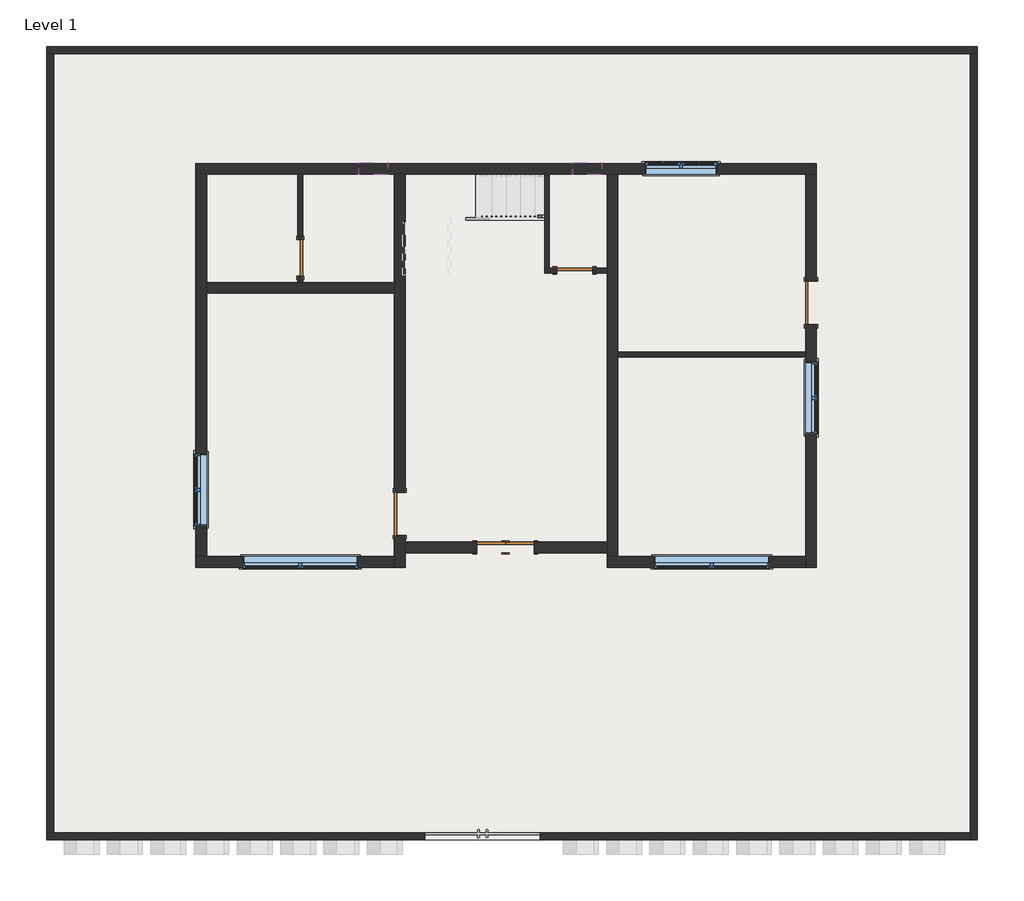
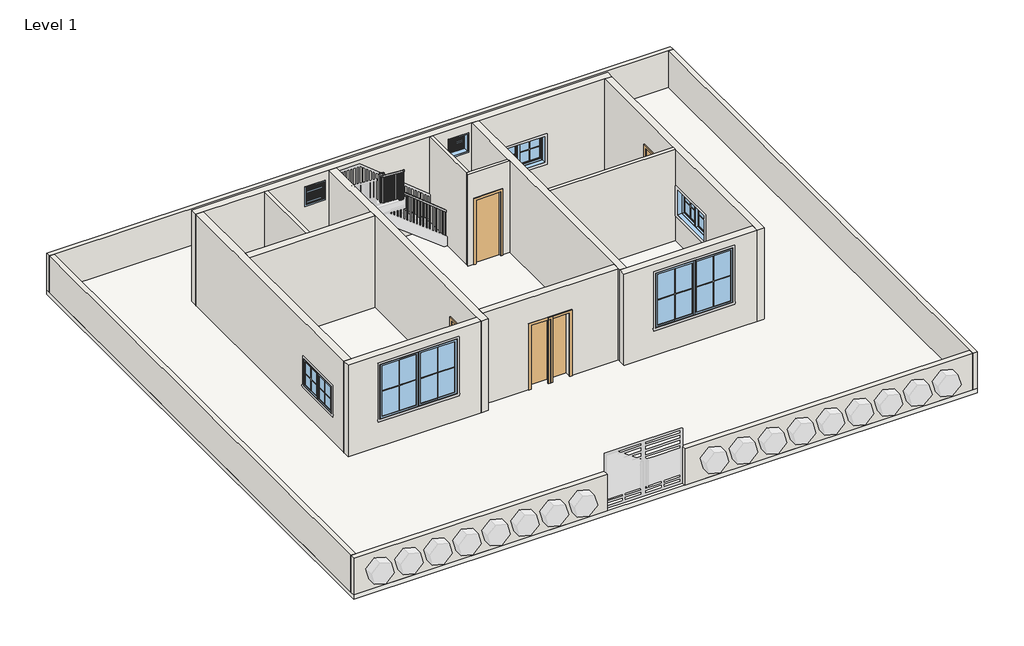
# One storey, part 1 of 2: 18 walls, 7 windows, 6 doors, 1 railing, 1 slab.
"""IFC4 building model written with IfcOpenShell, lengths in millimetres."""

from ifc_helpers import new_model, si_unit, frame, origin, origin_with_axes, place, context, project, spatial, polyline, outline, extrude, faceted_brep, transform, mapped, element, save
from components import single_flush_door_2_4a3212df, single_flush_door_2_0d3b4037, door_270f2424, door_aa9e95e7, single_flush_door_3_a90ba1ad, window_casement_double_c1d95f0f, window_casement_double_9ae172a2, window_f2d8fef0

model = new_model("IFC4")

# Units and contexts
model_context = context("Model", 3, world=origin())
ifc_project = project(units=[si_unit("LENGTHUNIT", "METRE", prefix="MILLI")], contexts=[model_context])

# Site, building, storey
site = spatial("IfcSite", under=ifc_project)
building = spatial("IfcBuilding", under=site)
storey = spatial("IfcBuildingStorey", under=building, Name="Level 1", Elevation=0.0)

# Doors
placement = place(None, origin())
single_flush_door_2_shape = single_flush_door_2_4a3212df(model_context)
element("IfcDoor", 1, ObjectType="Single-Flush : DOOR 2'", at=placement, inside=storey, context=model_context, shape_type="MappedRepresentation", body=[
    mapped(single_flush_door_2_shape, transform((-1572.7415084, -2604.3618005, 0.0), x_axis=(-1.0, 0.0, 0.0), y_axis=(0.0, -1.0, 0.0), z_axis=(0.0, 0.0, 1.0))),
])
single_flush_door_2_2_shape = single_flush_door_2_0d3b4037(model_context)
element("IfcDoor", 2, ObjectType="Single-Flush : DOOR 2'", at=placement, inside=storey, context=model_context, shape_type="MappedRepresentation", body=[
    mapped(single_flush_door_2_2_shape, transform((-963.1415084, -2604.3618005, 0.0), x_axis=(1.0, 0.0, 0.0), y_axis=(0.0, 1.0, 0.0), z_axis=(0.0, 0.0, 1.0))),
])
door_shape = door_270f2424(model_context)
element("IfcDoor", 3, ObjectType="Single-Flush : DOOR 2'6\"", at=placement, inside=storey, context=model_context, shape_type="MappedRepresentation", body=[
    mapped(door_shape, transform((-5598.6415084, 3517.0381995, 0.0), x_axis=(0.0, -1.0, 0.0), y_axis=(1.0, 0.0, 0.0), z_axis=(0.0, 0.0, 1.0))),
])
door_2_shape = door_aa9e95e7(model_context)
element("IfcDoor", 4, ObjectType="Single-Flush : DOOR 2'6\"", at=placement, inside=storey, context=model_context, shape_type="MappedRepresentation", body=[
    mapped(door_2_shape, transform((192.5584916, 3250.3381995, 0.0), x_axis=(-1.0, 0.0, 0.0), y_axis=(0.0, -1.0, 0.0), z_axis=(0.0, 0.0, 1.0))),
])
single_flush_door_3_shape = single_flush_door_3_a90ba1ad(model_context)
element("IfcDoor", 5, ObjectType="Single-Flush : DOOR 3'", at=placement, inside=storey, context=model_context, shape_type="MappedRepresentation", body=[
    mapped(single_flush_door_3_shape, transform((-3503.1415084, -1893.1618005, 0.0), x_axis=(0.0, -1.0, 0.0), y_axis=(1.0, 0.0, 0.0), z_axis=(0.0, 0.0, 1.0))),
])
element("IfcDoor", 6, ObjectType="Single-Flush : DOOR 3'", at=placement, inside=storey, context=model_context, shape_type="MappedRepresentation", body=[
    mapped(single_flush_door_3_shape, transform((5183.6584916, 2564.5381995, 0.0), x_axis=(0.0, -1.0, 0.0), y_axis=(1.0, 0.0, 0.0), z_axis=(0.0, 0.0, 1.0))),
])

# Railing
element("IfcRailing", 7, ObjectType="Handrail - Rectangular", at=placement, inside=storey, context=model_context, shape_type="SolidModel", body=[
    faceted_brep([(-442.4415084, 4368.3146777, 1148.8615385), (-442.4415084, 4368.3146777, 1083.5609717), (-442.4415084, 4419.1146777, 1083.5609717), (-442.4415084, 4419.1146777, 1148.8615385), (-2398.2415084, 4368.3146777, 2728.5461538), (-2449.0415084, 4368.3146777, 2704.2763563), (-2449.0415084, 4419.1146777, 2704.2763563), (-2398.2415084, 4419.1146777, 2728.5461538), (-2398.2415084, 4368.3146777, 3083.1511426), (-2449.0415084, 4368.3146777, 3032.3511426), (-2449.0415084, 4419.1146777, 3032.3511426), (-2398.2415084, 4419.1146777, 3083.1511426), (-2474.4415084, 4368.3146777, 3083.1511426), (-2474.4415084, 4368.3146777, 3032.3511426), (-2525.2415084, 4419.1146777, 3032.3511426), (-2525.2415084, 4419.1146777, 3083.1511426), (-2474.4415084, 4292.1146777, 3083.1511426), (-2474.4415084, 4274.8407094, 3032.3511426), (-2525.2415084, 4274.8407094, 3032.3511426), (-2525.2415084, 4292.1146777, 3083.1511426), (-2474.4415084, 3148.7383287, 3962.4), (-2525.2415084, 3148.7383287, 3962.4), (-2525.2415084, 3148.7383287, 3898.3164325), (-2474.4415084, 3148.7383287, 3898.3164325)], [[[0, 1, 2, 3]], [[1, 0, 4, 5]], [[2, 1, 5, 6]], [[3, 2, 6, 7]], [[0, 3, 7, 4]], [[5, 4, 8, 9]], [[6, 5, 9, 10]], [[7, 6, 10, 11]], [[4, 7, 11, 8]], [[9, 8, 12, 13]], [[10, 9, 13, 14]], [[11, 10, 14, 15]], [[8, 11, 15, 12]], [[13, 12, 16, 17]], [[14, 13, 17, 18]], [[15, 14, 18, 19]], [[12, 15, 19, 16]], [[20, 21, 22, 23]], [[17, 16, 20, 23]], [[18, 17, 23, 22]], [[19, 18, 22, 21]], [[16, 19, 21, 20]]]),
    extrude(outline(polyline([(3184.0396777, 3871.1699284), (3184.0396777, 2813.5384615), (3164.9896777, 2813.5384615), (3164.9896777, 3885.8192525), (3184.0396777, 3871.1699284)])), frame((-2509.3665084, 0.0, 0.0), z_axis=(1.0, 0.0, 0.0), x_axis=(0.0, 1.0, 0.0)), (0.0, 0.0, 1.0), 19.05),
    extrude(outline(polyline([(3285.6396777, 3793.0401997), (3285.6396777, 2813.5384615), (3266.5896777, 2813.5384615), (3266.5896777, 3807.6895238), (3285.6396777, 3793.0401997)])), frame((-2509.3665084, 0.0, 0.0), z_axis=(1.0, 0.0, 0.0), x_axis=(0.0, 1.0, 0.0)), (0.0, 0.0, 1.0), 19.05),
    extrude(outline(polyline([(3387.2396777, 3714.910471), (3387.2396777, 2813.5384615), (3368.1896777, 2813.5384615), (3368.1896777, 3729.5597952), (3387.2396777, 3714.910471)])), frame((-2509.3665084, 0.0, 0.0), z_axis=(1.0, 0.0, 0.0), x_axis=(0.0, 1.0, 0.0)), (0.0, 0.0, 1.0), 19.05),
    extrude(outline(polyline([(3488.8396777, 3636.9254473), (3488.8396777, 2579.0769231), (3469.7896777, 2579.0769231), (3469.7896777, 3651.5747714), (3488.8396777, 3636.9254473)])), frame((-2509.3665084, 0.0, 0.0), z_axis=(1.0, 0.0, 0.0), x_axis=(0.0, 1.0, 0.0)), (0.0, 0.0, 1.0), 19.05),
    extrude(outline(polyline([(3590.4396777, 3558.7957187), (3590.4396777, 2579.0769231), (3571.3896777, 2579.0769231), (3571.3896777, 3573.4450428), (3590.4396777, 3558.7957187)])), frame((-2509.3665084, 0.0, 0.0), z_axis=(1.0, 0.0, 0.0), x_axis=(0.0, 1.0, 0.0)), (0.0, 0.0, 1.0), 19.05),
    extrude(outline(polyline([(3692.0396777, 3480.66599), (3692.0396777, 2579.0769231), (3672.9896777, 2579.0769231), (3672.9896777, 3495.3153141), (3692.0396777, 3480.66599)])), frame((-2509.3665084, 0.0, 0.0), z_axis=(1.0, 0.0, 0.0), x_axis=(0.0, 1.0, 0.0)), (0.0, 0.0, 1.0), 19.05),
    extrude(outline(polyline([(3793.6396777, 3402.4639089), (3793.6396777, 2344.6153846), (3774.5896777, 2344.6153846), (3774.5896777, 3417.113233), (3793.6396777, 3402.4639089)])), frame((-2509.3665084, 0.0, 0.0), z_axis=(1.0, 0.0, 0.0), x_axis=(0.0, 1.0, 0.0)), (0.0, 0.0, 1.0), 19.05),
    extrude(outline(polyline([(3895.2396777, 3324.3341802), (3895.2396777, 2344.6153846), (3876.1896777, 2344.6153846), (3876.1896777, 3338.9835043), (3895.2396777, 3324.3341802)])), frame((-2509.3665084, 0.0, 0.0), z_axis=(1.0, 0.0, 0.0), x_axis=(0.0, 1.0, 0.0)), (0.0, 0.0, 1.0), 19.05),
    extrude(outline(polyline([(3996.8396777, 3246.2044515), (3996.8396777, 2344.6153846), (3977.7896777, 2344.6153846), (3977.7896777, 3260.8537757), (3996.8396777, 3246.2044515)])), frame((-2509.3665084, 0.0, 0.0), z_axis=(1.0, 0.0, 0.0), x_axis=(0.0, 1.0, 0.0)), (0.0, 0.0, 1.0), 19.05),
    extrude(outline(polyline([(4098.4396777, 3168.0023704), (4098.4396777, 2110.1538462), (4079.3896777, 2110.1538462), (4079.3896777, 3182.6516945), (4098.4396777, 3168.0023704)])), frame((-2509.3665084, 0.0, 0.0), z_axis=(1.0, 0.0, 0.0), x_axis=(0.0, 1.0, 0.0)), (0.0, 0.0, 1.0), 19.05),
    extrude(outline(polyline([(4200.0396777, 3089.8726417), (4200.0396777, 2110.1538462), (4180.9896777, 2110.1538462), (4180.9896777, 3104.5219659), (4200.0396777, 3089.8726417)])), frame((-2509.3665084, 0.0, 0.0), z_axis=(1.0, 0.0, 0.0), x_axis=(0.0, 1.0, 0.0)), (0.0, 0.0, 1.0), 19.05),
    extrude(outline(polyline([(4301.6396777, 3011.7429131), (4301.6396777, 2110.1538462), (4282.5896777, 2110.1538462), (4282.5896777, 3026.3922372), (4301.6396777, 3011.7429131)])), frame((-2509.3665084, 0.0, 0.0), z_axis=(1.0, 0.0, 0.0), x_axis=(0.0, 1.0, 0.0)), (0.0, 0.0, 1.0), 19.05),
    extrude(outline(polyline([(-2464.9165084, 4384.1896777), (-2483.9665084, 4384.1896777), (-2483.9665084, 4403.2396777), (-2464.9165084, 4403.2396777), (-2464.9165084, 4384.1896777)])), frame((0.0, 0.0, 1875.6923077), z_axis=(0.0, 0.0, 1.0), x_axis=(1.0, 0.0, 0.0)), (0.0, 0.0, 1.0), 1156.658835),
    extrude(outline(polyline([(2650.4234717, -2382.3665084), (1641.2307692, -2382.3665084), (1641.2307692, -2363.3165084), (2635.0369332, -2363.3165084), (2650.4234717, -2382.3665084)])), frame((0.0, 4384.1896777, 0.0), z_axis=(0.0, 1.0, 0.0), x_axis=(0.0, 0.0, 1.0)), (0.0, 0.0, 1.0), 19.05),
    extrude(outline(polyline([(2568.3619332, -2280.7665084), (1641.2307692, -2280.7665084), (1641.2307692, -2261.7165084), (2552.9753947, -2261.7165084), (2568.3619332, -2280.7665084)])), frame((0.0, 4384.1896777, 0.0), z_axis=(0.0, 1.0, 0.0), x_axis=(0.0, 0.0, 1.0)), (0.0, 0.0, 1.0), 19.05),
    extrude(outline(polyline([(2486.3003947, -2179.1665084), (1641.2307692, -2179.1665084), (1641.2307692, -2160.1165084), (2470.9138563, -2160.1165084), (2486.3003947, -2179.1665084)])), frame((0.0, 4384.1896777, 0.0), z_axis=(0.0, 1.0, 0.0), x_axis=(0.0, 0.0, 1.0)), (0.0, 0.0, 1.0), 19.05),
    extrude(outline(polyline([(2404.2388563, -2077.5665084), (1406.7692308, -2077.5665084), (1406.7692308, -2058.5165084), (2388.8523178, -2058.5165084), (2404.2388563, -2077.5665084)])), frame((0.0, 4384.1896777, 0.0), z_axis=(0.0, 1.0, 0.0), x_axis=(0.0, 0.0, 1.0)), (0.0, 0.0, 1.0), 19.05),
    extrude(outline(polyline([(2322.1773178, -1975.9665084), (1406.7692308, -1975.9665084), (1406.7692308, -1956.9165084), (2306.7907794, -1956.9165084), (2322.1773178, -1975.9665084)])), frame((0.0, 4384.1896777, 0.0), z_axis=(0.0, 1.0, 0.0), x_axis=(0.0, 0.0, 1.0)), (0.0, 0.0, 1.0), 19.05),
    extrude(outline(polyline([(2240.1157794, -1874.3665084), (1406.7692308, -1874.3665084), (1406.7692308, -1855.3165084), (2224.7292409, -1855.3165084), (2240.1157794, -1874.3665084)])), frame((0.0, 4384.1896777, 0.0), z_axis=(0.0, 1.0, 0.0), x_axis=(0.0, 0.0, 1.0)), (0.0, 0.0, 1.0), 19.05),
    extrude(outline(polyline([(2158.0542409, -1772.7665084), (1172.3076923, -1772.7665084), (1172.3076923, -1753.7165084), (2142.6677024, -1753.7165084), (2158.0542409, -1772.7665084)])), frame((0.0, 4384.1896777, 0.0), z_axis=(0.0, 1.0, 0.0), x_axis=(0.0, 0.0, 1.0)), (0.0, 0.0, 1.0), 19.05),
    extrude(outline(polyline([(2075.9927024, -1671.1665084), (1172.3076923, -1671.1665084), (1172.3076923, -1652.1165084), (2060.606164, -1652.1165084), (2075.9927024, -1671.1665084)])), frame((0.0, 4384.1896777, 0.0), z_axis=(0.0, 1.0, 0.0), x_axis=(0.0, 0.0, 1.0)), (0.0, 0.0, 1.0), 19.05),
    extrude(outline(polyline([(1993.931164, -1569.5665084), (1172.3076923, -1569.5665084), (1172.3076923, -1550.5165084), (1978.5446255, -1550.5165084), (1993.931164, -1569.5665084)])), frame((0.0, 4384.1896777, 0.0), z_axis=(0.0, 1.0, 0.0), x_axis=(0.0, 0.0, 1.0)), (0.0, 0.0, 1.0), 19.05),
    extrude(outline(polyline([(1911.8696255, -1467.9665084), (937.8461538, -1467.9665084), (937.8461538, -1448.9165084), (1896.4830871, -1448.9165084), (1911.8696255, -1467.9665084)])), frame((0.0, 4384.1896777, 0.0), z_axis=(0.0, 1.0, 0.0), x_axis=(0.0, 0.0, 1.0)), (0.0, 0.0, 1.0), 19.05),
    extrude(outline(polyline([(1829.8080871, -1366.3665084), (937.8461538, -1366.3665084), (937.8461538, -1347.3165084), (1814.4215486, -1347.3165084), (1829.8080871, -1366.3665084)])), frame((0.0, 4384.1896777, 0.0), z_axis=(0.0, 1.0, 0.0), x_axis=(0.0, 0.0, 1.0)), (0.0, 0.0, 1.0), 19.05),
    extrude(outline(polyline([(1747.7465486, -1264.7665084), (937.8461538, -1264.7665084), (937.8461538, -1245.7165084), (1732.3600101, -1245.7165084), (1747.7465486, -1264.7665084)])), frame((0.0, 4384.1896777, 0.0), z_axis=(0.0, 1.0, 0.0), x_axis=(0.0, 0.0, 1.0)), (0.0, 0.0, 1.0), 19.05),
    extrude(outline(polyline([(1665.6850101, -1163.1665084), (703.3846154, -1163.1665084), (703.3846154, -1144.1165084), (1650.2984717, -1144.1165084), (1665.6850101, -1163.1665084)])), frame((0.0, 4384.1896777, 0.0), z_axis=(0.0, 1.0, 0.0), x_axis=(0.0, 0.0, 1.0)), (0.0, 0.0, 1.0), 19.05),
    extrude(outline(polyline([(1583.6234717, -1061.5665084), (703.3846154, -1061.5665084), (703.3846154, -1042.5165084), (1568.2369332, -1042.5165084), (1583.6234717, -1061.5665084)])), frame((0.0, 4384.1896777, 0.0), z_axis=(0.0, 1.0, 0.0), x_axis=(0.0, 0.0, 1.0)), (0.0, 0.0, 1.0), 19.05),
    extrude(outline(polyline([(1501.5619332, -959.9665084), (703.3846154, -959.9665084), (703.3846154, -940.9165084), (1486.1753947, -940.9165084), (1501.5619332, -959.9665084)])), frame((0.0, 4384.1896777, 0.0), z_axis=(0.0, 1.0, 0.0), x_axis=(0.0, 0.0, 1.0)), (0.0, 0.0, 1.0), 19.05),
    extrude(outline(polyline([(1419.5003947, -858.3665084), (468.9230769, -858.3665084), (468.9230769, -839.3165084), (1404.1138563, -839.3165084), (1419.5003947, -858.3665084)])), frame((0.0, 4384.1896777, 0.0), z_axis=(0.0, 1.0, 0.0), x_axis=(0.0, 0.0, 1.0)), (0.0, 0.0, 1.0), 19.05),
    extrude(outline(polyline([(1337.4388563, -756.7665084), (468.9230769, -756.7665084), (468.9230769, -737.7165084), (1322.0523178, -737.7165084), (1337.4388563, -756.7665084)])), frame((0.0, 4384.1896777, 0.0), z_axis=(0.0, 1.0, 0.0), x_axis=(0.0, 0.0, 1.0)), (0.0, 0.0, 1.0), 19.05),
    extrude(outline(polyline([(1255.3773178, -655.1665084), (468.9230769, -655.1665084), (468.9230769, -636.1165084), (1239.9907794, -636.1165084), (1255.3773178, -655.1665084)])), frame((0.0, 4384.1896777, 0.0), z_axis=(0.0, 1.0, 0.0), x_axis=(0.0, 0.0, 1.0)), (0.0, 0.0, 1.0), 19.05),
    extrude(outline(polyline([(1173.3157794, -553.5665084), (234.4615385, -553.5665084), (234.4615385, -534.5165084), (1157.9292409, -534.5165084), (1173.3157794, -553.5665084)])), frame((0.0, 4384.1896777, 0.0), z_axis=(0.0, 1.0, 0.0), x_axis=(0.0, 0.0, 1.0)), (0.0, 0.0, 1.0), 19.05),
    extrude(outline(polyline([(-2490.3165084, 4384.1896777), (-2509.3665084, 4384.1896777), (-2509.3665084, 4403.2396777), (-2490.3165084, 4403.2396777), (-2490.3165084, 4384.1896777)])), frame((0.0, 0.0, 1875.6923077), z_axis=(0.0, 0.0, 1.0), x_axis=(1.0, 0.0, 0.0)), (0.0, 0.0, 1.0), 1156.658835),
    extrude(outline(polyline([(3167.7883287, 3883.6671084), (3167.7883287, 2813.5384615), (3148.7383287, 2813.5384615), (3148.7383287, 3898.3164325), (3167.7883287, 3883.6671084)])), frame((-2509.3665084, 0.0, 0.0), z_axis=(1.0, 0.0, 0.0), x_axis=(0.0, 1.0, 0.0)), (0.0, 0.0, 1.0), 19.05),
    extrude(outline(polyline([(1098.9475101, -461.4915084), (234.4615385, -461.4915084), (234.4615385, -442.4415084), (1083.5609717, -442.4415084), (1098.9475101, -461.4915084)])), frame((0.0, 4384.1896777, 0.0), z_axis=(0.0, 1.0, 0.0), x_axis=(0.0, 0.0, 1.0)), (0.0, 0.0, 1.0), 19.05),
])

# Slab
element("IfcSlab", 8, ObjectType="FLOOR 6\"", at=placement, inside=storey, context=model_context, shape_type="SweptSolid", body=[
    extrude(outline(polyline([(8700.0547931, 7982.1774536), (8700.0547931, -8781.8225464), (-10959.5452069, -8781.8225464), (-10959.5452069, 7982.1774536), (8700.0547931, 7982.1774536)])), frame((0.0, 0.0, -152.4), z_axis=(0.0, 0.0, 1.0), x_axis=(1.0, 0.0, 0.0)), (0.0, 0.0, 1.0), 152.4),
])

# Walls
element("IfcWall", 9, ObjectType="CMD 6\"", at=placement, inside=storey, context=model_context, shape_type="Brep", body=[
    faceted_brep([(-10959.5452069, 7829.7774536, 0.0), (-10807.1452069, 7829.7774536, 0.0), (8547.6547931, 7829.7774536, 0.0), (8700.0547931, 7829.7774536, 0.0), (8700.0547931, 7829.7774536, 1219.2), (8547.6547931, 7829.7774536, 1219.2), (-10807.1452069, 7829.7774536, 1219.2), (-10959.5452069, 7829.7774536, 1219.2), (-10959.5452069, 7982.1774536, 0.0), (-10959.5452069, 7982.1774536, 1219.2), (8700.0547931, 7982.1774536, 1219.2), (8700.0547931, 7982.1774536, 0.0)], [[[0, 1, 2, 3, 4, 5, 6, 7]], [[8, 9, 10, 11]], [[3, 2, 1, 0, 8, 11]], [[7, 6, 5, 4, 10, 9]], [[4, 3, 11, 10]], [[0, 7, 9, 8]]]),
])
element("IfcWall", 10, ObjectType="CMD 6\"", at=placement, inside=storey, context=model_context, shape_type="Brep", body=[
    faceted_brep([(8547.6547931, 7829.7774536, 0.0), (8547.6547931, -8629.4225464, 0.0), (8547.6547931, -8781.8225464, 0.0), (8547.6547931, -8781.8225464, 1219.2), (8547.6547931, -8629.4225464, 1219.2), (8547.6547931, 7829.7774536, 1219.2), (8700.0547931, 7829.7774536, 0.0), (8700.0547931, 7829.7774536, 1219.2), (8700.0547931, -8781.8225464, 1219.2), (8700.0547931, -8781.8225464, 0.0)], [[[0, 1, 2, 3, 4, 5]], [[6, 7, 8, 9]], [[2, 1, 0, 6, 9]], [[5, 4, 3, 8, 7]], [[0, 5, 7, 6]], [[3, 2, 9, 8]]]),
])
element("IfcWall", 11, ObjectType="CMD 6\"", at=placement, inside=storey, context=model_context, shape_type="SweptSolid", body=[
    extrude(outline(polyline([(-531.3415084, -8629.4225464), (8547.6547931, -8629.4225464), (8547.6547931, -8781.8225464), (-531.3415084, -8781.8225464), (-531.3415084, -8629.4225464)])), origin_with_axes(), (0.0, 0.0, 1.0), 1219.2),
])
element("IfcWall", 12, ObjectType="CMD 6\"", at=placement, inside=storey, context=model_context, shape_type="SweptSolid", body=[
    extrude(outline(polyline([(-10807.1452069, 7829.7774536), (-10807.1452069, -8629.4225464), (-10959.5452069, -8629.4225464), (-10959.5452069, 7829.7774536), (-10807.1452069, 7829.7774536)])), origin_with_axes(), (0.0, 0.0, 1.0), 1219.2),
])
element("IfcWall", 13, ObjectType="CMD 6\"", at=placement, inside=storey, context=model_context, shape_type="Brep", body=[
    faceted_brep([(-2969.7415084, -8629.4225464, 0.0), (-10807.1452069, -8629.4225464, 0.0), (-10959.5452069, -8629.4225464, 0.0), (-10959.5452069, -8629.4225464, 1219.2), (-10807.1452069, -8629.4225464, 1219.2), (-2969.7415084, -8629.4225464, 1219.2), (-2969.7415084, -8781.8225464, 0.0), (-2969.7415084, -8781.8225464, 1219.2), (-10959.5452069, -8781.8225464, 1219.2), (-10959.5452069, -8781.8225464, 0.0)], [[[0, 1, 2, 3, 4, 5]], [[6, 7, 8, 9]], [[2, 1, 0, 6, 9]], [[5, 4, 3, 8, 7]], [[0, 5, 7, 6]], [[3, 2, 9, 8]]]),
])
element("IfcWall", 14, ObjectType="WALL 4\"", at=placement, inside=storey, context=model_context, shape_type="SweptSolid", body=[
    extrude(outline(polyline([(3136.0381995, 2133.6), (3136.0381995, 0.0), (2996.3381995, 0.0), (2996.3381995, 3048.0), (5282.3381995, 3048.0), (5282.3381995, 0.0), (3898.0381995, 0.0), (3898.0381995, 2133.6), (3136.0381995, 2133.6)])), frame((-5649.4415084, 0.0, 0.0), z_axis=(1.0, 0.0, 0.0), x_axis=(0.0, 1.0, 0.0)), (0.0, 0.0, 1.0), 101.6),
])
element("IfcWall", 15, ObjectType="WALL 4\"", at=placement, inside=storey, context=model_context, shape_type="Brep", body=[
    faceted_brep([(-188.4415084, 3301.1381995, 2133.6), (-188.4415084, 3301.1381995, 0.0), (-340.8415084, 3301.1381995, 0.0), (-442.4415084, 3301.1381995, 0.0), (-442.4415084, 3301.1381995, 3048.0), (-340.8415084, 3301.1381995, 3048.0), (878.3584916, 3301.1381995, 3048.0), (878.3584916, 3301.1381995, 0.0), (573.5584916, 3301.1381995, 0.0), (573.5584916, 3301.1381995, 2133.6), (-442.4415084, 3199.5381995, 0.0), (-188.4415084, 3199.5381995, 0.0), (-188.4415084, 3199.5381995, 2133.6), (573.5584916, 3199.5381995, 2133.6), (573.5584916, 3199.5381995, 0.0), (878.3584916, 3199.5381995, 0.0), (878.3584916, 3199.5381995, 3048.0), (-442.4415084, 3199.5381995, 3048.0)], [[[0, 1, 2, 3, 4, 5, 6, 7, 8, 9]], [[10, 11, 12, 13, 14, 15, 16, 17]], [[8, 7, 15, 14]], [[3, 2, 1, 11, 10]], [[7, 6, 16, 15]], [[4, 3, 10, 17]], [[12, 11, 1, 0]], [[13, 12, 0, 9]], [[14, 13, 9, 8]], [[6, 5, 4, 17, 16]]]),
])
element("IfcWall", 16, ObjectType="WALL 4\"", at=placement, inside=storey, context=model_context, shape_type="Brep", body=[
    faceted_brep([(-340.8415084, 3301.1381995, 0.0), (-340.8415084, 5282.3381995, 0.0), (-340.8415084, 5282.3381995, 3048.0), (-340.8415084, 3301.1381995, 3048.0), (-442.4415084, 3301.1381995, 0.0), (-442.4415084, 3301.1381995, 3048.0), (-442.4415084, 4317.5146777, 3048.0), (-442.4415084, 5282.3381995, 3048.0), (-442.4415084, 5282.3381995, 0.0)], [[[0, 1, 2, 3]], [[4, 5, 6, 7, 8]], [[1, 0, 4, 8]], [[0, 3, 5, 4]], [[2, 1, 8, 7]], [[3, 2, 7, 6, 5]]]),
])
element("IfcWall", 17, ObjectType="WALL 4\"", at=placement, inside=storey, context=model_context, shape_type="SweptSolid", body=[
    extrude(outline(polyline([(1106.9584916, 1523.1381995), (5069.3584916, 1523.1381995), (5069.3584916, 1421.5381995), (1106.9584916, 1421.5381995), (1106.9584916, 1523.1381995)])), origin_with_axes(), (0.0, 0.0, 1.0), 3048.0),
])
element("IfcWall", 18, ObjectType="WALL 9\"", at=placement, inside=storey, context=model_context, shape_type="Brep", body=[
    faceted_brep([(-7808.4415084, 5282.3381995, 0.0), (-7579.8415084, 5282.3381995, 0.0), (-5649.4415084, 5282.3381995, 0.0), (-5547.8415084, 5282.3381995, 0.0), (-3617.4415084, 5282.3381995, 0.0), (-3388.8415084, 5282.3381995, 0.0), (-442.4415084, 5282.3381995, 0.0), (-340.8415084, 5282.3381995, 0.0), (878.3584916, 5282.3381995, 0.0), (1106.9584916, 5282.3381995, 0.0), (5069.3584916, 5282.3381995, 0.0), (5297.9584916, 5282.3381995, 0.0), (5297.9584916, 5282.3381995, 3048.0), (5069.3584916, 5282.3381995, 3048.0), (1106.9584916, 5282.3381995, 3048.0), (878.3584916, 5282.3381995, 3048.0), (-340.8415084, 5282.3381995, 3048.0), (-442.4415084, 5282.3381995, 3048.0), (-3388.8415084, 5282.3381995, 3048.0), (-3617.4415084, 5282.3381995, 3048.0), (-5547.8415084, 5282.3381995, 3048.0), (-5649.4415084, 5282.3381995, 3048.0), (-7579.8415084, 5282.3381995, 3048.0), (-7808.4415084, 5282.3381995, 3048.0), (3202.4584916, 5282.3381995, 1828.8), (3202.4584916, 5282.3381995, 914.4), (1678.4584916, 5282.3381995, 914.4), (1678.4584916, 5282.3381995, 1828.8), (154.4584916, 5282.3381995, 2743.2), (764.0584916, 5282.3381995, 2743.2), (764.0584916, 5282.3381995, 2133.6), (154.4584916, 5282.3381995, 2133.6), (-3757.1415084, 5282.3381995, 2743.2), (-3757.1415084, 5282.3381995, 2133.6), (-4366.7415084, 5282.3381995, 2133.6), (-4366.7415084, 5282.3381995, 2743.2), (-7808.4415084, 5510.9381995, 0.0), (-7808.4415084, 5510.9381995, 3048.0), (5297.9584916, 5510.9381995, 3048.0), (5297.9584916, 5510.9381995, 0.0), (3202.4584916, 5510.9381995, 1828.8), (1678.4584916, 5510.9381995, 1828.8), (1678.4584916, 5510.9381995, 914.4), (3202.4584916, 5510.9381995, 914.4), (154.4584916, 5510.9381995, 2743.2), (154.4584916, 5510.9381995, 2133.6), (764.0584916, 5510.9381995, 2133.6), (764.0584916, 5510.9381995, 2743.2), (-3757.1415084, 5510.9381995, 2743.2), (-4366.7415084, 5510.9381995, 2743.2), (-4366.7415084, 5510.9381995, 2133.6), (-3757.1415084, 5510.9381995, 2133.6)], [[[0, 1, 2, 3, 4, 5, 6, 7, 8, 9, 10, 11, 12, 13, 14, 15, 16, 17, 18, 19, 20, 21, 22, 23], [24, 25, 26, 27], [28, 29, 30, 31], [32, 33, 34, 35]], [[36, 37, 38, 39], [40, 41, 42, 43], [44, 45, 46, 47], [48, 49, 50, 51]], [[11, 10, 9, 8, 7, 6, 5, 4, 3, 2, 1, 0, 36, 39]], [[23, 22, 21, 20, 19, 18, 17, 16, 15, 14, 13, 12, 38, 37]], [[12, 11, 39, 38]], [[0, 23, 37, 36]], [[25, 24, 40, 43]], [[26, 25, 43, 42]], [[27, 26, 42, 41]], [[24, 27, 41, 40]], [[45, 44, 28, 31]], [[46, 45, 31, 30]], [[47, 46, 30, 29]], [[44, 47, 29, 28]], [[33, 32, 48, 51]], [[34, 33, 51, 50]], [[35, 34, 50, 49]], [[32, 35, 49, 48]]]),
])
element("IfcWall", 19, ObjectType="WALL 9\"", at=placement, inside=storey, context=model_context, shape_type="Brep", body=[
    faceted_brep([(5069.3584916, 2107.3381995, 2133.6), (5069.3584916, 2107.3381995, 0.0), (5069.3584916, 1523.1381995, 0.0), (5069.3584916, 1421.5381995, 0.0), (5069.3584916, -2794.8618005, 0.0), (5069.3584916, -3023.4618005, 0.0), (5069.3584916, -3023.4618005, 3048.0), (5069.3584916, -2794.8618005, 3048.0), (5069.3584916, 1421.5381995, 3048.0), (5069.3584916, 1523.1381995, 3048.0), (5069.3584916, 5282.3381995, 3048.0), (5069.3584916, 5282.3381995, 0.0), (5069.3584916, 3021.7381995, 0.0), (5069.3584916, 3021.7381995, 2133.6), (5069.3584916, -204.0618005, 1828.8), (5069.3584916, -204.0618005, 914.4), (5069.3584916, 1319.9381995, 914.4), (5069.3584916, 1319.9381995, 1828.8), (5297.9584916, -3023.4618005, 0.0), (5297.9584916, 2107.3381995, 0.0), (5297.9584916, 2107.3381995, 2133.6), (5297.9584916, 3021.7381995, 2133.6), (5297.9584916, 3021.7381995, 0.0), (5297.9584916, 5282.3381995, 0.0), (5297.9584916, 5282.3381995, 3048.0), (5297.9584916, -3023.4618005, 3048.0), (5297.9584916, -204.0618005, 1828.8), (5297.9584916, 1319.9381995, 1828.8), (5297.9584916, 1319.9381995, 914.4), (5297.9584916, -204.0618005, 914.4)], [[[0, 1, 2, 3, 4, 5, 6, 7, 8, 9, 10, 11, 12, 13], [14, 15, 16, 17]], [[18, 19, 20, 21, 22, 23, 24, 25], [26, 27, 28, 29]], [[12, 11, 23, 22]], [[5, 4, 3, 2, 1, 19, 18]], [[11, 10, 24, 23]], [[6, 5, 18, 25]], [[15, 14, 26, 29]], [[16, 15, 29, 28]], [[17, 16, 28, 27]], [[14, 17, 27, 26]], [[20, 19, 1, 0]], [[21, 20, 0, 13]], [[22, 21, 13, 12]], [[10, 9, 8, 7, 6, 25, 24]]]),
])
element("IfcWall", 20, ObjectType="WALL 9\"", at=placement, inside=storey, context=model_context, shape_type="Brep", body=[
    faceted_brep([(5069.3584916, -2794.8618005, 0.0), (1106.9584916, -2794.8618005, 0.0), (878.3584916, -2794.8618005, 0.0), (878.3584916, -2794.8618005, 3048.0), (1106.9584916, -2794.8618005, 3048.0), (5069.3584916, -2794.8618005, 3048.0), (1868.9584916, -2794.8618005, 2743.2), (1868.9584916, -2794.8618005, 914.4), (4307.3584916, -2794.8618005, 914.4), (4307.3584916, -2794.8618005, 2743.2), (5069.3584916, -3023.4618005, 0.0), (5069.3584916, -3023.4618005, 3048.0), (878.3584916, -3023.4618005, 3048.0), (878.3584916, -3023.4618005, 0.0), (1868.9584916, -3023.4618005, 2743.2), (4307.3584916, -3023.4618005, 2743.2), (4307.3584916, -3023.4618005, 914.4), (1868.9584916, -3023.4618005, 914.4)], [[[0, 1, 2, 3, 4, 5], [6, 7, 8, 9]], [[10, 11, 12, 13], [14, 15, 16, 17]], [[2, 1, 0, 10, 13]], [[0, 5, 11, 10]], [[3, 2, 13, 12]], [[7, 6, 14, 17]], [[8, 7, 17, 16]], [[9, 8, 16, 15]], [[6, 9, 15, 14]], [[5, 4, 3, 12, 11]]]),
])
element("IfcWall", 21, ObjectType="WALL 9\"", at=placement, inside=storey, context=model_context, shape_type="Brep", body=[
    faceted_brep([(1106.9584916, -2794.8618005, 0.0), (1106.9584916, 1421.5381995, 0.0), (1106.9584916, 1523.1381995, 0.0), (1106.9584916, 5282.3381995, 0.0), (1106.9584916, 5282.3381995, 3048.0), (1106.9584916, 1523.1381995, 3048.0), (1106.9584916, 1421.5381995, 3048.0), (1106.9584916, -2794.8618005, 3048.0), (878.3584916, -2794.8618005, 0.0), (878.3584916, -2794.8618005, 3048.0), (878.3584916, -2718.6618005, 3048.0), (878.3584916, -2490.0618005, 3048.0), (878.3584916, 3199.5381995, 3048.0), (878.3584916, 3301.1381995, 3048.0), (878.3584916, 5282.3381995, 3048.0), (878.3584916, 5282.3381995, 0.0), (878.3584916, 3301.1381995, 0.0), (878.3584916, 3199.5381995, 0.0), (878.3584916, -2490.0618005, 0.0), (878.3584916, -2718.6618005, 0.0)], [[[0, 1, 2, 3, 4, 5, 6, 7]], [[8, 9, 10, 11, 12, 13, 14, 15, 16, 17, 18, 19]], [[3, 2, 1, 0, 8, 19, 18, 17, 16, 15]], [[0, 7, 9, 8]], [[4, 3, 15, 14]], [[7, 6, 5, 4, 14, 13, 12, 11, 10, 9]]]),
])
element("IfcWall", 22, ObjectType="WALL 9\"", at=placement, inside=storey, context=model_context, shape_type="SweptSolid", body=[
    extrude(outline(polyline([(0.0, 878.3584916), (3048.0, 878.3584916), (3048.0, -3388.8415084), (0.0, -3388.8415084), (0.0, -1877.5415084), (2133.6, -1877.5415084), (2133.6, -658.3415084), (0.0, -658.3415084), (0.0, 878.3584916)])), frame((0.0, -2718.6618005, 0.0), z_axis=(0.0, 1.0, 0.0), x_axis=(0.0, 0.0, 1.0)), (0.0, 0.0, 1.0), 228.6),
])
element("IfcWall", 23, ObjectType="WALL 9\"", at=placement, inside=storey, context=model_context, shape_type="Brep", body=[
    faceted_brep([(-3388.8415084, -3023.4618005, 0.0), (-3388.8415084, -2718.6618005, 0.0), (-3388.8415084, -2490.0618005, 0.0), (-3388.8415084, -2350.3618005, 0.0), (-3388.8415084, -2350.3618005, 2133.6), (-3388.8415084, -1435.9618005, 2133.6), (-3388.8415084, -1435.9618005, 0.0), (-3388.8415084, 5282.3381995, 0.0), (-3388.8415084, 5282.3381995, 3048.0), (-3388.8415084, -2490.0618005, 3048.0), (-3388.8415084, -2718.6618005, 3048.0), (-3388.8415084, -3023.4618005, 3048.0), (-3617.4415084, -2350.3618005, 2133.6), (-3617.4415084, -2350.3618005, 0.0), (-3617.4415084, -2794.8618005, 0.0), (-3617.4415084, -3023.4618005, 0.0), (-3617.4415084, -3023.4618005, 3048.0), (-3617.4415084, -2794.8618005, 3048.0), (-3617.4415084, 2767.7381995, 3048.0), (-3617.4415084, 2996.3381995, 3048.0), (-3617.4415084, 5282.3381995, 3048.0), (-3617.4415084, 5282.3381995, 0.0), (-3617.4415084, 2996.3381995, 0.0), (-3617.4415084, 2767.7381995, 0.0), (-3617.4415084, -1435.9618005, 0.0), (-3617.4415084, -1435.9618005, 2133.6)], [[[0, 1, 2, 3, 4, 5, 6, 7, 8, 9, 10, 11]], [[12, 13, 14, 15, 16, 17, 18, 19, 20, 21, 22, 23, 24, 25]], [[15, 14, 13, 3, 2, 1, 0]], [[24, 23, 22, 21, 7, 6]], [[11, 10, 9, 8, 20, 19, 18, 17, 16]], [[8, 7, 21, 20]], [[0, 11, 16, 15]], [[4, 3, 13, 12]], [[5, 4, 12, 25]], [[6, 5, 25, 24]]]),
])
element("IfcWall", 24, ObjectType="WALL 9\"", at=placement, inside=storey, context=model_context, shape_type="Brep", body=[
    faceted_brep([(-3617.4415084, -2794.8618005, 0.0), (-7579.8415084, -2794.8618005, 0.0), (-7808.4415084, -2794.8618005, 0.0), (-7808.4415084, -2794.8618005, 3048.0), (-7579.8415084, -2794.8618005, 3048.0), (-3617.4415084, -2794.8618005, 3048.0), (-6817.8415084, -2794.8618005, 2743.2), (-6817.8415084, -2794.8618005, 914.4), (-4379.4415084, -2794.8618005, 914.4), (-4379.4415084, -2794.8618005, 2743.2), (-3617.4415084, -3023.4618005, 0.0), (-3617.4415084, -3023.4618005, 3048.0), (-7808.4415084, -3023.4618005, 3048.0), (-7808.4415084, -3023.4618005, 0.0), (-6817.8415084, -3023.4618005, 2743.2), (-4379.4415084, -3023.4618005, 2743.2), (-4379.4415084, -3023.4618005, 914.4), (-6817.8415084, -3023.4618005, 914.4)], [[[0, 1, 2, 3, 4, 5], [6, 7, 8, 9]], [[10, 11, 12, 13], [14, 15, 16, 17]], [[2, 1, 0, 10, 13]], [[0, 5, 11, 10]], [[3, 2, 13, 12]], [[7, 6, 14, 17]], [[8, 7, 17, 16]], [[9, 8, 16, 15]], [[6, 9, 15, 14]], [[5, 4, 3, 12, 11]]]),
])
element("IfcWall", 25, ObjectType="WALL 9\"", at=placement, inside=storey, context=model_context, shape_type="Brep", body=[
    faceted_brep([(-7579.8415084, -2794.8618005, 0.0), (-7579.8415084, 2767.7381995, 0.0), (-7579.8415084, 2996.3381995, 0.0), (-7579.8415084, 5282.3381995, 0.0), (-7579.8415084, 5282.3381995, 3048.0), (-7579.8415084, 2996.3381995, 3048.0), (-7579.8415084, 2767.7381995, 3048.0), (-7579.8415084, -2794.8618005, 3048.0), (-7579.8415084, -623.1618005, 1828.8), (-7579.8415084, -623.1618005, 914.4), (-7579.8415084, -2147.1618005, 914.4), (-7579.8415084, -2147.1618005, 1828.8), (-7808.4415084, -2794.8618005, 0.0), (-7808.4415084, -2794.8618005, 3048.0), (-7808.4415084, 5282.3381995, 3048.0), (-7808.4415084, 5282.3381995, 0.0), (-7808.4415084, -623.1618005, 1828.8), (-7808.4415084, -2147.1618005, 1828.8), (-7808.4415084, -2147.1618005, 914.4), (-7808.4415084, -623.1618005, 914.4)], [[[0, 1, 2, 3, 4, 5, 6, 7], [8, 9, 10, 11]], [[12, 13, 14, 15], [16, 17, 18, 19]], [[3, 2, 1, 0, 12, 15]], [[0, 7, 13, 12]], [[4, 3, 15, 14]], [[9, 8, 16, 19]], [[10, 9, 19, 18]], [[11, 10, 18, 17]], [[8, 11, 17, 16]], [[7, 6, 5, 4, 14, 13]]]),
])
element("IfcWall", 26, ObjectType="WALL 9\"", at=placement, inside=storey, context=model_context, shape_type="Brep", body=[
    faceted_brep([(-7579.8415084, 2767.7381995, 0.0), (-3617.4415084, 2767.7381995, 0.0), (-3617.4415084, 2767.7381995, 3048.0), (-7579.8415084, 2767.7381995, 3048.0), (-7579.8415084, 2996.3381995, 0.0), (-7579.8415084, 2996.3381995, 3048.0), (-5649.4415084, 2996.3381995, 3048.0), (-5547.8415084, 2996.3381995, 3048.0), (-3617.4415084, 2996.3381995, 3048.0), (-3617.4415084, 2996.3381995, 0.0), (-5547.8415084, 2996.3381995, 0.0), (-5649.4415084, 2996.3381995, 0.0)], [[[0, 1, 2, 3]], [[4, 5, 6, 7, 8, 9, 10, 11]], [[1, 0, 4, 11, 10, 9]], [[2, 1, 9, 8]], [[0, 3, 5, 4]], [[3, 2, 8, 7, 6, 5]]]),
])

# Windows
window_casement_double_shape = window_casement_double_c1d95f0f(model_context)
element("IfcWindow", 27, ObjectType="Window-Casement-Double", at=placement, inside=storey, context=model_context, shape_type="MappedRepresentation", body=[
    mapped(window_casement_double_shape, transform((-7694.1415084, -1385.1618005, 0.0), x_axis=(0.0, 1.0, 0.0), y_axis=(-1.0, 0.0, 0.0), z_axis=(0.0, 0.0, 1.0))),
])
element("IfcWindow", 28, ObjectType="Window-Casement-Double", at=placement, inside=storey, context=model_context, shape_type="MappedRepresentation", body=[
    mapped(window_casement_double_shape, transform((5183.6584916, 557.9381995, 0.0), x_axis=(0.0, -1.0, 0.0), y_axis=(1.0, 0.0, 0.0), z_axis=(0.0, 0.0, 1.0))),
])
element("IfcWindow", 29, ObjectType="Window-Casement-Double", at=placement, inside=storey, context=model_context, shape_type="MappedRepresentation", body=[
    mapped(window_casement_double_shape, transform((2440.4584916, 5396.6381995, 0.0), x_axis=(1.0, 0.0, 0.0), y_axis=(0.0, 1.0, 0.0), z_axis=(0.0, 0.0, 1.0))),
])
window_casement_double_2_shape = window_casement_double_9ae172a2(model_context)
element("IfcWindow", 30, ObjectType="Window-Casement-Double", at=placement, inside=storey, context=model_context, shape_type="MappedRepresentation", body=[
    mapped(window_casement_double_2_shape, transform((-5598.6415084, -2909.1618005, 0.0), x_axis=(-1.0, 0.0, 0.0), y_axis=(0.0, -1.0, 0.0), z_axis=(0.0, 0.0, 1.0))),
])
element("IfcWindow", 31, ObjectType="Window-Casement-Double", at=placement, inside=storey, context=model_context, shape_type="MappedRepresentation", body=[
    mapped(window_casement_double_2_shape, transform((3088.1584916, -2909.1618005, 0.0), x_axis=(-1.0, 0.0, 0.0), y_axis=(0.0, -1.0, 0.0), z_axis=(0.0, 0.0, 1.0))),
])
window_shape = window_f2d8fef0(model_context)
element("IfcWindow", 32, ObjectType="Window-Louvers : 24\" x 24\"", at=placement, inside=storey, context=model_context, shape_type="MappedRepresentation", body=[
    mapped(window_shape, transform((459.2584916, 5402.9881995, 1219.2), x_axis=(1.0, 0.0, 0.0), y_axis=(0.0, 1.0, 0.0), z_axis=(0.0, 0.0, 1.0))),
])
element("IfcWindow", 33, ObjectType="Window-Louvers : 24\" x 24\"", at=placement, inside=storey, context=model_context, shape_type="MappedRepresentation", body=[
    mapped(window_shape, transform((-4061.9415084, 5390.2881995, 1219.2), x_axis=(-1.0, 0.0, 0.0), y_axis=(0.0, -1.0, 0.0), z_axis=(0.0, 0.0, 1.0))),
])

save(model, "model.ifc")

# Revit data of these elements
# Type "Single-Flush : DOOR 2'"
#   Type Mark = "10"
#   Construction Type Id = "MDOOR"
#   Assembly Code = "C1020"
#   Analytic Construction = "Metal"
#   Thickness = 0' - 2"
#   Heat Transfer Coefficient (U) = 0.651978 BTU/(h·ft²·°F)
#   Height = 7' - 0"
#   Trim Projection Ext = 0' - 1"
#   Trim Projection Int = 0' - 1"
#   Trim Width = 0' - 3"
#   Width = 2' - 0"
#   Define Thermal Properties by = 1
#   Door Material = Door - Panel
#   Frame Material = Door - Frame
#   Visual Light Transmittance = 0
#   Solar Heat Gain Coefficient = 0
#   Function = (empty or 0)
#   Wall Closure = (empty or 0)
# Type "Single-Flush : DOOR 2'6\""
#   Type Mark = "9"
#   Construction Type Id = "MDOOR"
#   Assembly Code = "C1020"
#   Analytic Construction = "Metal"
#   Thickness = 0' - 2"
#   Heat Transfer Coefficient (U) = 0.651978 BTU/(h·ft²·°F)
#   Height = 7' - 0"
#   Trim Projection Ext = 0' - 1"
#   Trim Projection Int = 0' - 1"
#   Trim Width = 0' - 3"
#   Width = 2' - 6"
#   Define Thermal Properties by = 1
#   Door Material = Door - Panel
#   Frame Material = Door - Frame
#   Visual Light Transmittance = 0
#   Solar Heat Gain Coefficient = 0
#   Function = (empty or 0)
#   Wall Closure = (empty or 0)
# Type "Single-Flush : DOOR 3'"
#   Type Mark = "8"
#   Construction Type Id = "MDOOR"
#   Assembly Code = "C1020"
#   Analytic Construction = "Metal"
#   Thickness = 0' - 2"
#   Heat Transfer Coefficient (U) = 0.651978 BTU/(h·ft²·°F)
#   Height = 7' - 0"
#   Trim Projection Ext = 0' - 1"
#   Trim Projection Int = 0' - 1"
#   Trim Width = 0' - 3"
#   Width = 3' - 0"
#   Define Thermal Properties by = 1
#   Door Material = Door - Panel
#   Frame Material = Door - Frame
#   Visual Light Transmittance = 0
#   Solar Heat Gain Coefficient = 0
#   Function = (empty or 0)
#   Wall Closure = (empty or 0)
# Type "Handrail - Rectangular"
#   Assembly Code = "C2010400"
#   built-in parameter 1008612 = 0.0416667 (stored number, unit not read)
#   built-in parameter 1008611 = 0.0416667 (stored number, unit not read)
#   built-in parameter 1008609 = 0.333333 (stored number, unit not read)
#   built-in parameter 1008604 = 0.166667 (stored number, unit not read)
#   built-in parameter 1008603 = 0.166667 (stored number, unit not read)
#   Railing Height = 3' - 0"
#   built-in parameter 1008630 = 2
#   built-in parameter 1008610 = 2
#   built-in parameter 1008618 = Baluster - Square : 3/4"
# Type "FLOOR 6\""
#   Assembly Code = "B1010"
#   Function = 0
#   Layers, outside or top first: 0' - 6" no material (function 1)
# Type "CMD 6\""
#   Assembly Code = "B2010"
#   Layers, outside or top first: 0' - 6" no material (function 1)
# Type "WALL 4\""
#   Assembly Code = "B2010"
#   Layers, outside or top first: 0' - 4" no material (function 1)
# Type "WALL 9\""
#   Assembly Code = "B2010"
#   Layers, outside or top first: 0' - 9" no material (function 1)
# Type "Window-Casement-Double"
#   Type Mark = "18"
#   Fire Rating = "0.5h"
#   Assembly Code = "B2020100"
#   Analytic Construction = "Double glazing - domestic"
#   Frame Extension [instance default] = 0' - 0 1/4"
#   Window Inset [instance default] = 0' - 0"
#   Wall Thickness [instance default] = 0' - 6"
#   Interior Wall Closure [instance default] = 0' - 2 1/4"
#   Half Width = 2' - 6"
#   Visual Light Transmittance = 0.81
#   Thermal Resistance (R) = 1.8146 (h·ft²·°F)/BTU
#   Solar Heat Gain Coefficient = 0.76
#   Rough Width = 5' - 0 1/2"
#   Rough Height = 3' - 0 1/2"
#   Height = 3' - 0"
#   Heat Transfer Coefficient (U) = 0.5511 BTU/(h·ft²·°F)
#   Exterior Wall Closure [instance default] = 0' - 1 1/4"
#   Extension Jamb [instance default] = 0' - 2 1/4"
#   Default Sill Height = 3' - 0"
#   Width = 5' - 0"
#   Muntin Visibility = yes
#   Interior Trim Visibility [instance default] = yes
#   Exterior Trim Visibility [instance default] = yes
#   Extension Jamb Visibility [instance default] = yes
#   Interior Trim Material = Wood - Stained
#   Muntin Pattern = Muntin Pattern_2x2 : Muntin Pattern_2x2
#   Interior Trim = Trim-Window-Interior-Flat : Picture Frame
#   Interior Frame Material = Wood - Stained
#   Glass Panel Material = Glass
#   Exterior Trim Material = Clad - White
#   Exterior Trim = Trim-Window-Exterior-Flat : with Sill
#   Exterior Frame Material = Clad - White
#   Wall Closure = (empty or 0)
# Type "Window-Casement-Double"
#   Type Mark = "19"
#   Fire Rating = "0.5h"
#   Assembly Code = "B2020100"
#   Analytic Construction = "Double glazing - domestic"
#   Frame Extension [instance default] = 0' - 0 1/4"
#   Window Inset [instance default] = 0' - 0"
#   Wall Thickness [instance default] = 0' - 6"
#   Interior Wall Closure [instance default] = 0' - 2 1/4"
#   Half Width = 4' - 0"
#   Visual Light Transmittance = 0.81
#   Thermal Resistance (R) = 1.8146 (h·ft²·°F)/BTU
#   Solar Heat Gain Coefficient = 0.76
#   Rough Width = 8' - 0 1/2"
#   Rough Height = 6' - 0 1/2"
#   Height = 6' - 0"
#   Heat Transfer Coefficient (U) = 0.5511 BTU/(h·ft²·°F)
#   Exterior Wall Closure [instance default] = 0' - 1 1/4"
#   Extension Jamb [instance default] = 0' - 2 1/4"
#   Default Sill Height = 3' - 0"
#   Width = 8' - 0"
#   Muntin Visibility = yes
#   Interior Trim Visibility [instance default] = yes
#   Exterior Trim Visibility [instance default] = yes
#   Extension Jamb Visibility [instance default] = yes
#   Interior Trim Material = Wood - Stained
#   Muntin Pattern = Muntin Pattern_2x2 : Muntin Pattern_2x2
#   Interior Trim = Trim-Window-Interior-Flat : Picture Frame
#   Interior Frame Material = Wood - Stained
#   Glass Panel Material = Glass
#   Exterior Trim Material = Clad - White
#   Exterior Trim = Trim-Window-Exterior-Flat : with Sill
#   Exterior Frame Material = Clad - White
#   Wall Closure = (empty or 0)
# Type "Window-Louvers : 24\" x 24\""
#   Type Mark = "20"
#   Construction Type Id = "GSP4R"
#   Assembly Code = "B20"
#   Analytic Construction = "1/8 in Pilkington single glazing"
#   Visual Light Transmittance = 0.9
#   Thermal Resistance (R) = 1.53941 (h·ft²·°F)/BTU
#   Solar Heat Gain Coefficient = 0.78
#   Max Height = 1' - 11.74264"
#   Height = 2' - 0"
#   Heat Transfer Coefficient (U) = 0.6496 BTU/(h·ft²·°F)
#   Blade Width [instance default] = 1' - 10 1/2"
#   Blade Vertical Thickness = 0' - 0.35355"
#   Blade Thickness = 0' - 0 1/4"
#   Blade Spacing = 0' - 1 1/2"
#   Blade Height = 0' - 1.85355"
#   Blade Depth = 0' - 3"
#   Blade Angle = 45.00°
#   Default Sill Height = 3' - 0"
#   Trim Projection_Exterior = 0' - 0 1/2"
#   Trim Projection_Interior = 0' - 0 1/2"
#   Trim Width_Exterior = 0' - 1 1/2"
#   Trim Width_Interior = 0' - 1 1/2"
#   Width = 2' - 0"
#   Max Blade Count = 12
#   Define Thermal Properties by = 1
#   Blade Count = 12
#   Frame Material = Birch
#   Louver Material = Birch
#   Trim Exterior Material = Birch
#   Trim Interior Material = Birch
#   Wall Closure = (empty or 0)
# Elements 1, 2 (IfcDoor, "Single-Flush : DOOR 2'")
#   Phase Created = New Construction
#   Materials on its faces: "Door - Frame", "Door - Panel"
# Elements 3, 4 (IfcDoor, "Single-Flush : DOOR 2'6\"")
#   Phase Created = New Construction
#   Materials on its faces: "Door - Frame", "Door - Panel"
# Elements 5, 6 (IfcDoor, "Single-Flush : DOOR 3'")
#   Phase Created = New Construction
#   Materials on its faces: "Door - Frame", "Door - Panel"
# Element 7 (IfcRailing, "Handrail - Rectangular")
#   Phase Created = New Construction
# Element 8 (IfcSlab, "FLOOR 6\"")
#   Height Offset From Level = 0' - 0"
#   Phase Created = New Construction
#   Materials on its faces: "Door - Frame", "Clad - White", "Wood - Stained"
# Element 9 (IfcWall, "CMD 6\"")
#   Top Offset = 0' - 0"
#   Base Offset = 0' - 0"
#   Unconnected Height = 4' - 0"
#   wall height = 4' - 0"
#   Phase Created = New Construction
#   Base Constraint = Level 1
#   Materials on its faces: "Clad - White", "Door - Frame"
# Elements 10, 13 (IfcWall, "CMD 6\"")
#   Top Offset = 0' - 0"
#   Base Offset = 0' - 0"
#   Unconnected Height = 4' - 0"
#   wall height = 4' - 0"
#   Phase Created = New Construction
#   Base Constraint = Level 1
#   Materials on its faces: "Clad - White", "Default Wall", "Door - Frame"
# Elements 11, 12 (IfcWall, "CMD 6\"")
#   Top Offset = 0' - 0"
#   Base Offset = 0' - 0"
#   Unconnected Height = 4' - 0"
#   wall height = 4' - 0"
#   Phase Created = New Construction
#   Base Constraint = Level 1
#   Materials on its faces: "Default Wall", "Clad - White", "Door - Frame"
# Elements 14, 17 (IfcWall, "WALL 4\"")
#   Top Offset = 0' - 0"
#   Base Offset = 0' - 0"
#   Unconnected Height = 10' - 0"
#   wall height = 10' - 0"
#   Phase Created = New Construction
#   Base Constraint = Level 1
#   Materials on its faces: "Default Wall"
# Elements 15, 16 (IfcWall, "WALL 4\"")
#   Top Offset = 0' - 0"
#   Base Offset = 0' - 0"
#   Unconnected Height = 10' - 0"
#   wall height = 10' - 0"
#   Phase Created = New Construction
#   Base Constraint = Level 1
#   Materials on its faces: "Default Wall", "Door - Frame"
# Element 18 (IfcWall, "WALL 9\"")
#   Top Offset = 0' - 0"
#   Base Offset = 0' - 0"
#   Unconnected Height = 10' - 0"
#   wall height = 10' - 0"
#   Phase Created = New Construction
#   Base Constraint = Level 1
#   Materials on its faces: "Default Wall", "Parking Stripe", "Door - Frame"
# Elements 19, 20, 21, 22, 24, 25 (IfcWall, "WALL 9\"")
#   Top Offset = 0' - 0"
#   Base Offset = 0' - 0"
#   Unconnected Height = 10' - 0"
#   wall height = 10' - 0"
#   Phase Created = New Construction
#   Base Constraint = Level 1
#   Materials on its faces: "Default Wall", "Parking Stripe"
# Element 23 (IfcWall, "WALL 9\"")
#   Top Offset = 0' - 0"
#   Base Offset = 0' - 0"
#   Unconnected Height = 10' - 0"
#   wall height = 10' - 0"
#   Phase Created = New Construction
#   Base Constraint = Level 1
#   Materials on its faces: "Default Wall", "Door - Frame", "Parking Stripe"
# Element 26 (IfcWall, "WALL 9\"")
#   Top Offset = 0' - 0"
#   Base Offset = 0' - 0"
#   Unconnected Height = 10' - 0"
#   wall height = 10' - 0"
#   Phase Created = New Construction
#   Base Constraint = Level 1
#   Materials on its faces: "Default Wall"
# Element 27 (IfcWindow, "Window-Casement-Double")
#   Mark = "1"
#   Window Inset = 0' - 0"
#   Interior Wall Closure = 0' - 2 1/4"
#   Frame Extension = 0' - 0 1/4"
#   Exterior Wall Closure = 0' - 1 1/4"
#   Interior Trim Visibility = yes
#   Exterior Trim Visibility = yes
#   Phase Created = New Construction
#   Materials on its faces: "Wood - Stained", "Glass", "Clad - White"
# Element 28 (IfcWindow, "Window-Casement-Double")
#   Mark = "2"
#   Window Inset = 0' - 0"
#   Interior Wall Closure = 0' - 2 1/4"
#   Frame Extension = 0' - 0 1/4"
#   Exterior Wall Closure = 0' - 1 1/4"
#   Interior Trim Visibility = yes
#   Exterior Trim Visibility = yes
#   Phase Created = New Construction
#   Materials on its faces: "Wood - Stained", "Glass", "Clad - White"
# Element 29 (IfcWindow, "Window-Casement-Double")
#   Mark = "3"
#   Window Inset = 0' - 0"
#   Interior Wall Closure = 0' - 2 1/4"
#   Frame Extension = 0' - 0 1/4"
#   Exterior Wall Closure = 0' - 1 1/4"
#   Interior Trim Visibility = yes
#   Exterior Trim Visibility = yes
#   Phase Created = New Construction
#   Materials on its faces: "Wood - Stained", "Glass", "Clad - White"
# Element 30 (IfcWindow, "Window-Casement-Double")
#   Mark = "4"
#   Window Inset = 0' - 0"
#   Interior Wall Closure = 0' - 2 1/4"
#   Frame Extension = 0' - 0 1/4"
#   Exterior Wall Closure = 0' - 1 1/4"
#   Interior Trim Visibility = yes
#   Exterior Trim Visibility = yes
#   Phase Created = New Construction
#   Materials on its faces: "Wood - Stained", "Glass", "Clad - White"
# Element 31 (IfcWindow, "Window-Casement-Double")
#   Mark = "5"
#   Window Inset = 0' - 0"
#   Interior Wall Closure = 0' - 2 1/4"
#   Frame Extension = 0' - 0 1/4"
#   Exterior Wall Closure = 0' - 1 1/4"
#   Interior Trim Visibility = yes
#   Exterior Trim Visibility = yes
#   Phase Created = New Construction
#   Materials on its faces: "Wood - Stained", "Glass", "Clad - White"
# Element 32 (IfcWindow, "Window-Louvers : 24\" x 24\"")
#   Mark = "6"
#   Blade Width = 1' - 10 1/2"
#   Phase Created = New Construction
#   Materials on its faces: "Birch"
# Element 33 (IfcWindow, "Window-Louvers : 24\" x 24\"")
#   Mark = "7"
#   Blade Width = 1' - 10 1/2"
#   Phase Created = New Construction
#   Materials on its faces: "Birch"
# Materials
#   "Door - Panel": class "Wood", colour RGB 210 159 95, transparency 0, Cost = 0
#   "Door - Frame": colour RGB 118 70 51, transparency 0, Cost = 0
#   "Wood - Stained": class "Wood", colour RGB 224 178 126, transparency 0, Cost = 0
#   "Glass": class "Glass", colour RGB 0 128 192, transparency 0.75, Description = "Soda Lime Glass", Cost = 0
#   "Clad - White": class "Wood", colour RGB 242 242 238, transparency 0, Cost = 0
#   "Birch": class "Wood", colour RGB 224 178 126, transparency 0, Description = "Betula Alleghaniensis", Cost = 0
#   "Default Wall": colour RGB 128 128 128, transparency 0, Cost = 0
#   "Parking Stripe": class "Paint", colour RGB 250 250 91, transparency 0, Cost = 0
